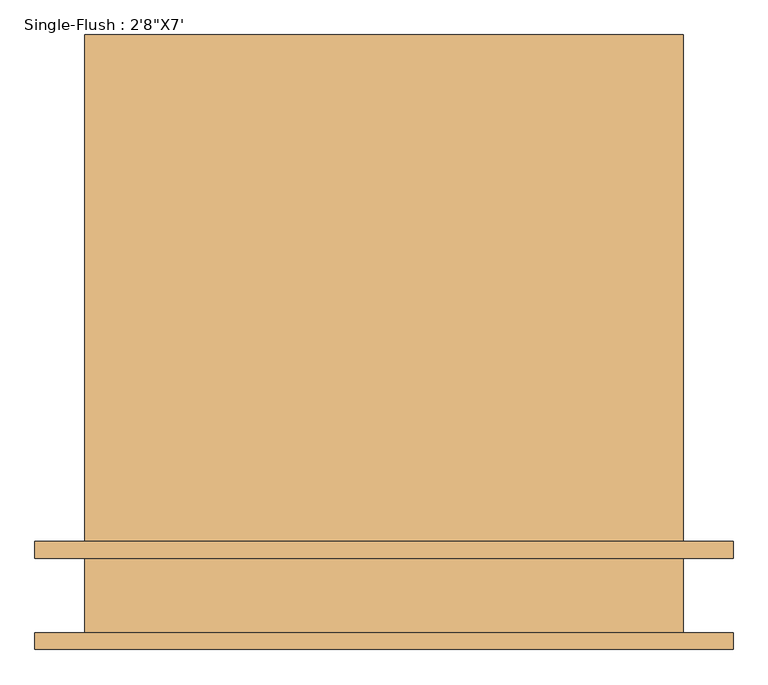
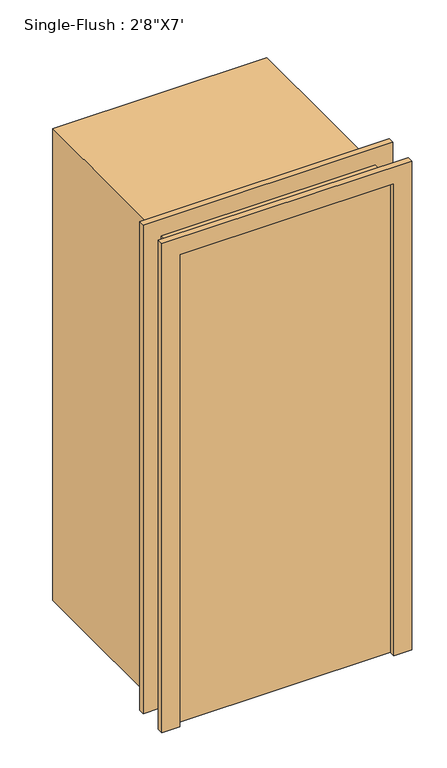
"""IFC4 building model written with IfcOpenShell, lengths in millimetres: door geometry."""

from ifc_helpers import new_model, si_unit, frame, origin, origin_with_axes, place, context, project, spatial, polyline, outline, extrude, source, transform, mapped, element, save


def door_0dbedf7e(model_context):
    return source(origin(), model_context, "Body", "SweptSolid", [
        extrude(outline(polyline([(2209.8, -533.4), (0.0, -533.4), (0.0, -457.2), (2133.6, -457.2), (2133.6, 457.2), (0.0, 457.2), (0.0, 533.4), (2209.8, 533.4), (2209.8, -533.4)])), frame((0.0, -82.55, 0.0), z_axis=(0.0, 1.0, 0.0), x_axis=(0.0, 0.0, 1.0)), (0.0, 0.0, 1.0), 25.4),
        extrude(outline(polyline([(2209.8, 533.4), (2209.8, -533.4), (0.0, -533.4), (0.0, -457.2), (2133.6, -457.2), (2133.6, 457.2), (0.0, 457.2), (0.0, 533.4), (2209.8, 533.4)])), frame((0.0, 57.15, 0.0), z_axis=(0.0, 1.0, 0.0), x_axis=(0.0, 0.0, 1.0)), (0.0, 0.0, 1.0), 25.4),
        extrude(outline(polyline([(457.2, 857.25), (457.2, -57.15), (-457.2, -57.15), (-457.2, 857.25), (457.2, 857.25)])), origin_with_axes(), (0.0, 0.0, 1.0), 2133.6),
    ])


if __name__ == "__main__":
    model = new_model("IFC4")
    model_context = context("Model", 3, world=origin())
    ifc_project = project(units=[si_unit("LENGTHUNIT", "METRE", prefix="MILLI")], contexts=[model_context])
    site = spatial("IfcSite", under=ifc_project)
    building = spatial("IfcBuilding", under=site)
    placement = place(None, origin())
    door_shape = door_0dbedf7e(model_context)
    element("IfcDoor", 1, ObjectType="Single-Flush : 2'8\"X7'", at=placement, inside=building, context=model_context, shape_type="MappedRepresentation", body=[
        mapped(door_shape, transform((0.0, 0.0, 0.0), x_axis=(1.0, 0.0, 0.0), y_axis=(0.0, 1.0, 0.0), z_axis=(0.0, 0.0, 1.0))),
    ])
    save(model, "model.ifc")

# Revit data of these elements
# Type "Single-Flush : 2'8\"X7'"
#   Type Mark = "8"
#   Construction Type Id = "MDOOR"
#   Assembly Code = "C1020"
#   Analytic Construction = "Metal"
#   Thickness = 3' - 0"
#   Heat Transfer Coefficient (U) = 0.651978 BTU/(h·ft²·°F)
#   Height = 7' - 0"
#   Trim Projection Ext = 0' - 1"
#   Trim Projection Int = 0' - 1"
#   Trim Width = 0' - 3"
#   Width = 3' - 0"
#   Define Thermal Properties by = 1
#   Door Material = Door - Panel
#   Frame Material = Door - Frame
#   Visual Light Transmittance = 0
#   Solar Heat Gain Coefficient = 0
#   Function = (empty or 0)
#   Wall Closure = (empty or 0)
# Element 1 (IfcDoor, "Single-Flush : 2'8\"X7'")
#   Materials on its faces: "Door - Frame", "Door - Panel"
# Materials
#   "Door - Panel": class "Wood", colour RGB 210 159 95, transparency 0, Cost = 0
#   "Door - Frame": colour RGB 118 70 51, transparency 0, Cost = 0
